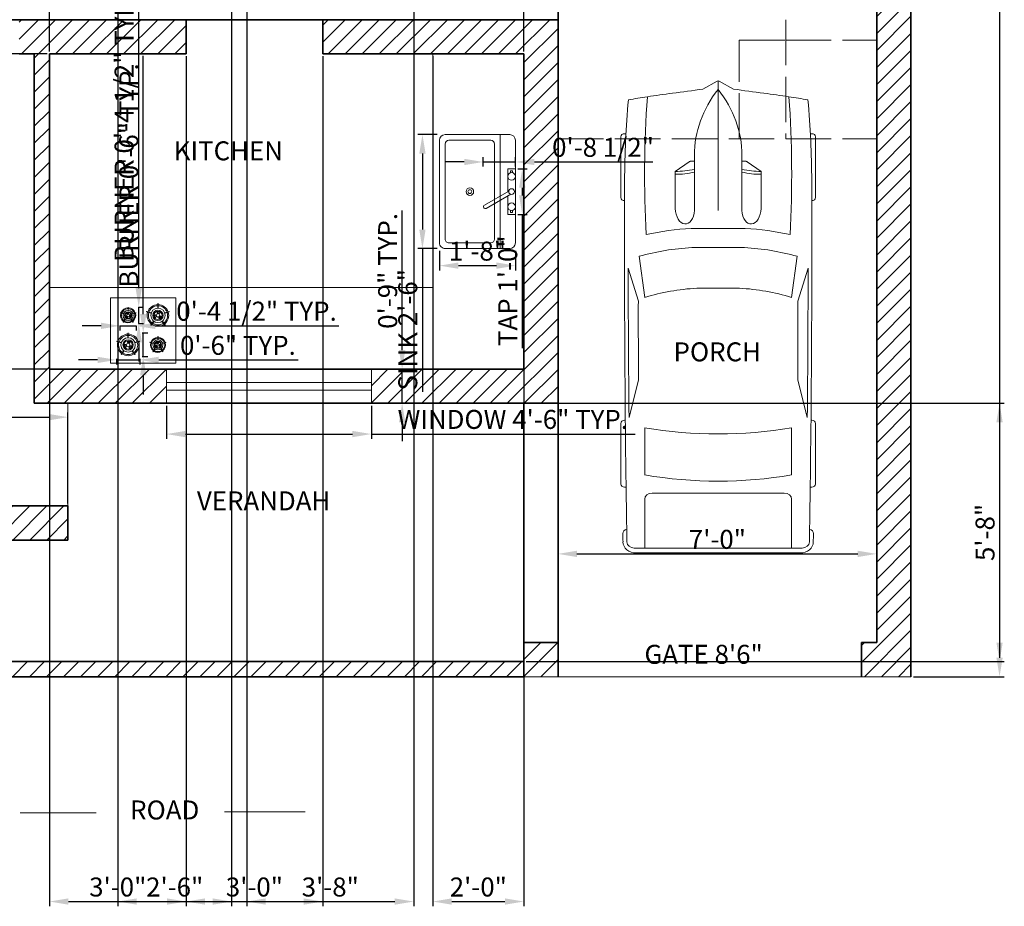
# Model space of a CAD drawing. Units: inches. Extents: x -33 to 381, y -443 to 47.
# Tile 3 of 5: x 122 to 381, y -443 to -210. Entities that reach past the tile are written whole.
import ezdxf

# ---------------------------------------------------------------- set-up
doc = ezdxf.new("R2010")
doc.units = ezdxf.units.IN
doc.linetypes.add('ACAD_ISO02W100', pattern=[15, 12, -3])
for name, color, linetype, lineweight in [('A-ANNO-DIMS', 2, 'Continuous', 18), ('A-ANNO-SYMB', 7, 'Continuous', 18), ('A-ANNO-TEXT', 7, 'Continuous', 18), ('A-AREA-IDEN', 7, 'Continuous', 18), ('A-DOOR', 4, 'Continuous', 18), ('A-EQPM', 8, 'Continuous', 15), ('A-FLOR-CASE', 9, 'Continuous', 18), ('A-FLOR-FIXT', 9, 'Continuous', 18), ('A-FLOR-STRS-OVHD', 8, 'ACAD_ISO02W100', 13), ('A-GLAZ', 4, 'Continuous', 18), ('A-SITE-VEHI', 8, 'Continuous', 13), ('A-WALL', 7, 'Continuous', 35), ('A-WALL-PATT', 251, 'Continuous', 13)]:
    doc.layers.add(name, color=color, linetype=linetype, lineweight=lineweight)
doc.styles.get("Standard").update_dxf_attribs({"font": 'arial.ttf'})
doc.dimstyles.new('ISO-25', dxfattribs={"dimtxt": 5, "dimasz": 5, "dimexe": 1.25, "dimexo": 0.625, "dimtad": 1, "dimlunit": 3, "dimtxsty": 'Standard', "dimcen": 2.5, "dimadec": 0, "dimazin": 0, "dimtfac": 1, "dimtmove": 0, "dimatfit": 3, "dimfxl": 1, "dimarcsym": 0})
pattern_1 = [(45, (-607.8963, -64.2963), (-2.245064, 2.245064), [])]

# ---------------------------------------------------------------- blocks, each defined once
blk = doc.blocks.new('Sink-single - 30 in top')
blk.add_line((-15, -3.999996), (15, -3.999996))
for points in [[(-13.5, 0), (13.5, 0)], [(-15, -18.499996), (-15, -1.5)], [(15, -1.5), (15, -18.499996)], [(-13.5, -17.499996), (-13.5, -6.499996)], [(-12.5, -5.499996), (12.5, -5.499996)], [(13.5, -6.499996), (13.5, -17.499996)], [(13.5, -19.999996), (-13.5, -19.999996)], [(12.5, -18.499996), (-12.5, -18.499996)]]:
    blk.add_lwpolyline(points)
for radius in [1, 0.5]:
    blk.add_circle((0, -11.999996), radius)
for centre, radius, start, end in [((-13.5, -1.5), 1.5, 90, 180), ((13.5, -1.5), 1.5, 0, 90), ((-12.5, -6.499996), 1, 90, 180), ((12.5, -6.499996), 1, 0, 90), ((-12.5, -17.499996), 1, 180, 270), ((12.5, -17.499996), 1, 270, 0), ((-13.5, -18.499996), 1.5, 180, 270), ((13.5, -18.499996), 1.5, 270, 0)]:
    blk.add_arc(centre, radius, start, end)
blk = doc.blocks.new('Faucet - kit sink top')
for p, q in [((-5.5, -0.75), (-5.5, -1.25)), ((-4.94278, -0.75), (-5.5, -0.75)), ((-5.5, -1.25), (-4.94278, -1.25)), ((-0.14775, -1.7441), (3.56698, -8.1782)), ((4.43301, -7.6782), (0.71828, -1.2441)), ((4.94278, -0.75), (5.5, -0.75)), ((5.5, -1.25), (4.94278, -1.25)), ((5.5, -0.75), (5.5, -1.25))]:
    blk.add_line(p, q)
blk.add_lwpolyline([(-0.00587, -2), (-6, -2), (-6, 0), (6, 0), (6, -2), (1.15195, -2)])
for centre, radius in [((-4, -1), 1), ((4, -1), 1), ((0, -1), 0.75)]:
    blk.add_circle(centre, radius)
blk.add_arc((4, -7.9282), 0.5, 210, 30)
blk = doc.blocks.new('*U10')
for p, q in [((21.1, 37.41), (21.1, 36.83)), ((46.55, 38.89), (22.35, 38.89)), ((47.8, 37.39), (47.8, 37.41)), ((87.99, 31.87), (74.76, 35.92)), ((134.31, 35.6), (119.29, 31.78)), ((135.45, 37.07), (135.45, 37.41)), ((136.7, 38.89), (160.9, 38.89)), ((162.15, 37.41), (162.15, 36.77)), ((70.03, 31.54), (86.41, 29.35)), ((186.47, -33.5), (186.47, 33.5)), ((188.4, -32.76), (188.4, 32.76)), ((138.42, 29.35), (157.25, 29.35)), ((186.47, 29.35), (167.01, 29.35)), ((164.52, 26.39), (164.52, -26.39)), ((32.27, 11.63), (36.13, 17.17)), ((36.13, 17.17), (50.94, 17.17)), ((29.77, 9.51), (51.68, 9.51)), ((32.12, 9.51), (32.12, 11.15)), ((58.92, -10.77), (58.92, 10.77)), ((66.55, -10.53), (66.55, 10.53)), ((82.74, 8.5), (82.74, -8.5)), ((186.47, -10.53), (186.47, 10.53)), ((3.27, 6.13), (0.1, 0.41)), ((0, 0), (51.68, 0)), ((0.1, -0.41), (3.27, -6.13)), ((29.77, -9.51), (51.68, -9.51)), ((32.12, -9.51), (32.12, -11.15)), ((32.27, -11.63), (36.13, -17.17)), ((36.13, -17.17), (50.94, -17.17)), ((86.41, -29.35), (70.03, -31.54)), ((157.25, -29.35), (138.42, -29.35)), ((167.01, -29.35), (186.47, -29.35)), ((87.99, -31.87), (74.76, -35.92)), ((134.31, -35.6), (119.29, -31.78)), ((21.1, -37.41), (21.1, -36.83)), ((46.55, -38.89), (22.35, -38.89)), ((47.8, -37.39), (47.8, -37.41)), ((135.45, -37.07), (135.45, -37.41)), ((136.7, -38.89), (160.9, -38.89)), ((162.15, -37.41), (162.15, -36.77))]:
    blk.add_line(p, q)
for centre, major_axis, ratio, start_param, end_param in [((266.03, -27.52), (0, 313.31), 0.842304, 1.367076, 1.39176), ((41.19, -490.86), (0, 528.23), 0.842304, 0.00281, 0.075598), ((22.35, 37.41), (0, -1.48), 0.842304, 3.141593, 4.712389), ((64.48, -10555.62), (0, 10593.03), 0.842304, -0.013397, 0.002797), ((46.55, 37.41), (0, 1.48), 0.842304, -1.570796, 0), ((64.48, -10555.62), (0, -10591.55), 0.842304, 3.133765, 3.140441), ((136.7, 37.41), (0, -1.48), 0.842304, 3.141593, 4.712389), ((160.9, 37.41), (0, 1.48), 0.842304, -1.570796, 0), ((180.63, 35.84), (0, 2.22), 0.842304, -0.013017, 1.249894), ((64.48, -10556.36), (0, 10595.31), 0.842304, -0.013397, -0.013017), ((183.98, 33.5), (0, -2.96), 0.842304, 1.570796, 3.128196), ((183.98, 32.76), (0, -5.25), 0.842304, 1.570796, 3.128196), ((135.29, 5.39), (0, 81.77), 0.842304, 1.245306, 1.50788), ((95.79, -3666.35), (0, -3698.24), 0.842304, 3.134049, 3.144098), ((259.18, -27.52), (0, -305.3), 0.842304, 4.528606, 4.561838), ((37.47, -593.96), (0, -623.33), 0.842304, 3.096046, 3.200911), ((134.4, 5.39), (0, -89.78), 0.842304, 4.449482, 4.652344), ((149.6, 2.8), (0, -79.58), 0.842304, 4.372215, 4.640744), ((17.08, 0), (0, 147.02), 0.842304, 4.511394, 4.913384), ((35.91, 0), (0, 147.02), 0.842304, 4.511394, 4.913384), ((167.01, 26.39), (0, 2.96), 0.842304, 0, 1.570796), ((-204.49, 52.4), (0, -250.96), 0.842304, 1.385369, 1.434372), ((13.04, 17.01), (0, 27.42), 0.842304, 4.435146, 4.718221), ((14.2, 17.01), (0, 27.42), 0.842304, 4.435146, 4.718221), ((50.79, 13.34), (6.34, -0.36), 0.603834, -1.395552, 1.581315), ((29.77, -46.66), (0, 56.17), 0.842304, 0, 0.590319), ((32.75, 11.15), (0, 0.74), 0.842304, 0.879714, 1.570796), ((0.62, 0), (0, -0.74), 0.842304, 4.131459, 5.293319), ((29.77, 46.66), (0, 56.17), 0.842304, 2.551274, 3.141593), ((-204.49, -52.4), (0, 250.96), 0.842304, -1.434372, -1.385369), ((32.75, -11.15), (0, -0.74), 0.842304, 4.712389, 5.403472), ((13.04, -17.01), (0, -27.42), 0.842304, 1.564964, 1.848039), ((14.2, -17.01), (0, -27.42), 0.842304, 1.564964, 1.848039), ((134.4, -5.39), (0, -89.78), 0.842304, -1.510751, -1.307889), ((135.29, -5.39), (0, -81.77), 0.842304, -1.50788, -1.245306), ((149.6, -2.8), (0, -79.58), 0.842304, -1.499151, -1.230623), ((259.18, 27.52), (0, 305.3), 0.842304, 1.721348, 1.754579), ((167.01, -26.39), (0, -2.96), 0.842304, 4.712389, 6.283185), ((266.03, 27.52), (0, 313.31), 0.842304, 1.749832, 1.774517), ((37.47, 593.96), (0, -623.33), 0.842304, -0.059319, 0.045547), ((95.79, 3666.35), (0, -3698.24), 0.842304, -0.002505, 0.007544), ((183.98, -33.5), (0, 2.96), 0.842304, 3.15499, 4.712389), ((183.98, -32.76), (0, -5.25), 0.842304, 0.013397, 1.570796), ((41.19, 490.86), (0, -528.23), 0.842304, -0.075598, -0.00281), ((22.35, -37.41), (0, 1.48), 0.842304, 1.570796, 3.141593), ((64.48, 10555.62), (0, 10593.03), 0.842304, 3.138796, 3.15499), ((46.55, -37.41), (0, -1.48), 0.842304, 0, 1.570796), ((64.48, 10555.62), (0, -10591.55), 0.842304, 0.001152, 0.007828), ((136.7, -37.41), (0, -1.48), 0.842304, -1.570796, 0), ((160.9, -37.41), (0, 1.48), 0.842304, 3.141593, 4.712389), ((180.63, -35.84), (0, -2.22), 0.842304, -1.249894, 0.013017), ((64.48, 10556.36), (0, 10595.31), 0.842304, 3.15461, 3.15499)]:
    blk.add_ellipse(centre, major_axis=major_axis, ratio=ratio, start_param=start_param, end_param=end_param)
at = {"extrusion": (0, 0, -1)}
blk.add_ellipse((50.79, -13.34), major_axis=(6.34, 0.36), ratio=0.603834, start_param=-1.395552, end_param=1.581315, dxfattribs=at)
blk = doc.blocks.new('COOKTOP-BURNER-LARGE')
for p, q in [((2.95, 4.78), (2.95, 5.94)), ((3.05, 4.78), (3.05, 5.94)), ((1.14, 3.39), (0.03, 3.75)), ((1.17, 3.48), (0.06, 3.84)), ((4.83, 3.48), (5.94, 3.84)), ((4.86, 3.39), (5.97, 3.75)), ((1.82, 1.3), (1.14, 0.35)), ((1.9, 1.24), (1.21, 0.3)), ((4.1, 1.24), (4.78, 0.3)), ((4.18, 1.3), (4.86, 0.35))]:
    blk.add_line(p, q)
for radius in [1.89, 1.36, 1.1, 0.473]:
    blk.add_circle((3, 2.84), radius)
for centre, radius, start, end in [((3, 2.84), 2.84, 90.9557, 161.0457), ((3, 2.84), 2.52, 91.075, 160.9263), ((3, 5.94), 0.0473, 0.0007, 180.0007), ((3, 2.84), 2.84, 18.9557, 89.0457), ((3, 2.84), 2.52, 19.075, 88.9263), ((0.05, 3.8), 0.0473, 72.0007, 252.0007), ((3, 2.84), 2.84, 162.9557, 233.0457), ((3, 2.84), 2.52, 163.075, 232.9263), ((1.15, 3.44), 0.0473, 252.0007, 72.0007), ((2.21, 2.84), 0.158, 0.0007, 180.0007), ((3, 2.84), 0.946, 180.0007, 213.5265), ((3, 2.84), 0.631, 180.0007, 213.5265), ((2.95, 3.62), 0.158, 93.5265, 273.5265), ((3, 2.84), 0.946, 60.0007, 93.5265), ((3, 4.78), 0.0473, 180.0007, 0.0007), ((3, 2.84), 0.631, 60.0007, 93.5265), ((3.39, 3.52), 0.158, 240.0007, 60.0007), ((3.7, 2.49), 0.158, 333.5265, 153.5265), ((3, 2.84), 2.52, 307.075, 16.9263), ((3, 2.84), 2.84, 306.9557, 17.0457), ((4.84, 3.44), 0.0473, 108.0007, 288.0007), ((5.95, 3.8), 0.0473, 288.0007, 108.0007), ((1.17, 0.33), 0.0473, 144.0007, 324.0007), ((3, 2.84), 2.84, 234.9557, 305.0457), ((3, 2.84), 2.52, 235.075, 304.9263), ((1.86, 1.27), 0.0473, 324.0007, 144.0007), ((2.34, 2.4), 0.158, 213.5265, 33.5265), ((3.39, 2.16), 0.158, 120.0007, 300.0007), ((3, 2.84), 0.631, 300.0007, 333.5265), ((3, 2.84), 0.946, 300.0007, 333.5265), ((4.14, 1.27), 0.0473, 36.0007, 216.0007), ((4.82, 0.33), 0.0473, 216.0007, 36.0007)]:
    blk.add_arc(centre, radius, start, end)
blk = doc.blocks.new('COOKTOP-BURNER-SMALL')
for p, q in [((0.8, 2.37), (0.02, 2.63)), ((0.82, 2.44), (0.04, 2.69)), ((2.07, 3.34), (2.07, 4.16)), ((2.13, 3.34), (2.13, 4.16)), ((3.38, 2.44), (4.15, 2.69)), ((3.4, 2.37), (4.18, 2.63)), ((1.27, 0.91), (0.8, 0.25)), ((1.33, 0.87), (0.85, 0.21)), ((2.87, 0.87), (3.35, 0.21)), ((2.92, 0.91), (3.4, 0.25))]:
    blk.add_line(p, q)
for radius in [1.32, 0.949, 0.772, 0.331]:
    blk.add_circle((2.1, 1.99), radius)
for centre, radius, start, end in [((0.03, 2.66), 0.0331, 72.0007, 252.0007), ((2.1, 1.99), 1.99, 90.9557, 161.0457), ((2.1, 1.99), 1.77, 91.075, 160.9263), ((2.1, 1.99), 0.662, 86.4748, 120.0007), ((2.1, 4.16), 0.0331, 0.0007, 180.0007), ((2.1, 3.34), 0.0331, 180.0007, 0.0007), ((2.1, 1.99), 1.99, 18.9557, 89.0457), ((2.1, 1.99), 1.77, 19.075, 88.9263), ((2.13, 2.54), 0.11, 266.4748, 86.4748), ((4.17, 2.66), 0.0331, 288.0007, 108.0007), ((2.1, 1.99), 1.99, 162.9557, 233.0457), ((2.1, 1.99), 1.77, 163.075, 232.9263), ((0.82, 0.23), 0.0331, 144.0007, 324.0007), ((0.81, 2.41), 0.0331, 252.0007, 72.0007), ((2.02, 1.99), 1.99, 234.9557, 305.0457), ((2.1, 1.99), 1.77, 235.075, 304.9263), ((1.3, 0.89), 0.0331, 324.0007, 144.0007), ((1.61, 1.74), 0.11, 26.4748, 206.4748), ((2.1, 1.99), 0.662, 206.4748, 240.0007), ((2.1, 1.99), 0.441, 206.4748, 240.0007), ((1.82, 2.46), 0.11, 120.0007, 300.0007), ((1.82, 1.51), 0.11, 240.0007, 60.0007), ((2.1, 1.99), 0.441, 86.4748, 120.0007), ((2.56, 1.68), 0.11, 146.4748, 326.4748), ((2.1, 1.99), 0.441, 326.4748, 0.0007), ((2.65, 1.99), 0.11, 0.0007, 180.0007), ((2.1, 1.99), 0.662, 326.4748, 0.0007), ((2.9, 0.89), 0.0331, 36.0007, 216.0007), ((2.1, 1.99), 1.77, 307.075, 16.9263), ((2.1, 1.99), 1.99, 306.9557, 17.0457), ((3.38, 0.23), 0.0331, 216.0007, 36.0007), ((3.39, 2.41), 0.0331, 108.0007, 288.0007)]:
    blk.add_arc(centre, radius, start, end)
blk = doc.blocks.new('WINDOW-54IN')
for p, q in [((0, 5.5), (54, 5.5)), ((0, 3.5), (54, 3.5))]:
    blk.add_line(p, q)
blk.add_lwpolyline([(0, 9), (54, 9), (54, 0), (0, 0)], close=True)
blk = doc.blocks.new('*D27')
at = {"layer": 'A-ANNO-DIMS', "color": 0, "lineweight": -2, "transparency": 16777216}
for p, q in [((160.37, -311.45), (160.37, -320.17)), ((214.37, -311.45), (214.37, -320.17)), ((165.37, -318.92), (209.37, -318.92)), ((214.37, -318.92), (283.9, -318.92))]:
    blk.add_line(p, q, dxfattribs=at)
at = {"layer": 'A-ANNO-DIMS', "color": 0, "transparency": 16777216}
for points in [[(165.37, -318.09), (165.37, -319.75), (160.37, -318.92)], [(209.37, -318.09), (209.37, -319.75), (214.37, -318.92)]]:
    blk.add_solid(points, dxfattribs=at)
at = {"layer": 'Defpoints', "color": 0, "transparency": 16777216}
for p in [(160.37, -310.82), (214.37, -310.82), (214.37, -318.92)]:
    blk.add_point(p, dxfattribs=at)
at = {"layer": 'A-ANNO-DIMS', "color": 0, "transparency": 16777216, "insert": (251.63, -315.71), "char_height": 5, "attachment_point": 5}
blk.add_mtext('WINDOW 4\'-6" TYP.', dxfattribs=at)
blk = doc.blocks.new('*D28')
at = {"layer": 'A-ANNO-DIMS', "color": 0, "lineweight": -2, "transparency": 16777216}
for p, q in [((222.47, -296.82), (222.47, -260.09)), ((215, -301.82), (223.72, -301.82)), ((222.47, -310.82), (222.47, -301.82)), ((215, -310.82), (223.72, -310.82)), ((222.47, -315.82), (222.47, -320.82))]:
    blk.add_line(p, q, dxfattribs=at)
at = {"layer": 'A-ANNO-DIMS', "color": 0, "transparency": 16777216}
for points in [[(221.64, -296.82), (223.31, -296.82), (222.47, -301.82)], [(221.64, -315.82), (223.31, -315.82), (222.47, -310.82)]]:
    blk.add_solid(points, dxfattribs=at)
at = {"layer": 'Defpoints', "color": 0, "transparency": 16777216}
for p in [(214.37, -301.82), (222.47, -301.82), (214.37, -310.82)]:
    blk.add_point(p, dxfattribs=at)
at = {"layer": 'A-ANNO-DIMS', "color": 0, "transparency": 16777216, "insert": (219.3, -275.96), "char_height": 5, "attachment_point": 5, "rotation": 90}
blk.add_mtext('0\'-9" TYP.', dxfattribs=at)
blk = doc.blocks.new('*D31')
at = {"layer": 'A-ANNO-DIMS', "color": 0, "lineweight": -2, "transparency": 16777216}
for p, q in [((231.69, -240.08), (226.57, -240.08)), ((227.82, -245.08), (227.82, -265.08)), ((231.69, -270.08), (226.57, -270.08)), ((227.82, -270.08), (227.82, -307.84))]:
    blk.add_line(p, q, dxfattribs=at)
at = {"layer": 'A-ANNO-DIMS', "color": 0, "transparency": 16777216}
for points in [[(226.98, -245.08), (228.65, -245.08), (227.82, -240.08)], [(226.98, -265.08), (228.65, -265.08), (227.82, -270.08)]]:
    blk.add_solid(points, dxfattribs=at)
at = {"layer": 'Defpoints', "color": 0, "transparency": 16777216}
for p in [(232.32, -240.08), (227.82, -270.08), (232.32, -270.08)]:
    blk.add_point(p, dxfattribs=at)
at = {"layer": 'A-ANNO-DIMS', "color": 0, "transparency": 16777216, "insert": (224.6, -291.46), "char_height": 5, "attachment_point": 5, "rotation": 90}
blk.add_mtext('SINK 2\'-6"', dxfattribs=at)
blk = doc.blocks.new('*D32')
at = {"layer": 'A-ANNO-DIMS', "color": 0, "lineweight": -2, "transparency": 16777216}
for p, q in [((232.32, -270.7), (232.32, -275.83)), ((252.32, -270.7), (252.32, -275.83)), ((237.32, -274.58), (247.32, -274.58))]:
    blk.add_line(p, q, dxfattribs=at)
at = {"layer": 'A-ANNO-DIMS', "color": 0, "transparency": 16777216}
for points in [[(237.32, -273.74), (237.32, -275.41), (232.32, -274.58)], [(247.32, -273.74), (247.32, -275.41), (252.32, -274.58)]]:
    blk.add_solid(points, dxfattribs=at)
at = {"layer": 'Defpoints', "color": 0, "transparency": 16777216}
for p in [(232.32, -270.08), (252.32, -270.08), (252.32, -274.58)]:
    blk.add_point(p, dxfattribs=at)
at = {"layer": 'A-ANNO-DIMS', "color": 0, "transparency": 16777216, "insert": (242.32, -271.4), "char_height": 5, "attachment_point": 5}
blk.add_mtext('1\'-8"', dxfattribs=at)
blk = doc.blocks.new('*D33')
at = {"layer": 'A-ANNO-DIMS', "color": 0, "lineweight": -2, "transparency": 16777216}
for p, q in [((252.94, -249.08), (255.37, -249.08)), ((254.12, -254.08), (254.12, -256.08)), ((252.94, -261.08), (255.37, -261.08)), ((254.12, -261.08), (254.12, -296.27))]:
    blk.add_line(p, q, dxfattribs=at)
at = {"layer": 'A-ANNO-DIMS', "color": 0, "transparency": 16777216}
for points in [[(253.28, -254.08), (254.95, -254.08), (254.12, -249.08)], [(253.28, -256.08), (254.95, -256.08), (254.12, -261.08)]]:
    blk.add_solid(points, dxfattribs=at)
at = {"layer": 'Defpoints', "color": 0, "transparency": 16777216}
for p in [(252.32, -249.08), (252.32, -261.08), (254.12, -261.08)]:
    blk.add_point(p, dxfattribs=at)
at = {"layer": 'A-ANNO-DIMS', "color": 0, "transparency": 16777216, "insert": (250.94, -281.17), "char_height": 5, "attachment_point": 5, "rotation": 90}
blk.add_mtext('TAP 1\'-0"', dxfattribs=at)
blk = doc.blocks.new('*D34')
at = {"layer": 'A-ANNO-DIMS', "color": 0, "lineweight": -2, "transparency": 16777216}
for p, q in [((243.82, -248.45), (243.82, -246.03)), ((252.32, -248.45), (252.32, -246.03)), ((238.82, -247.28), (233.82, -247.28)), ((243.82, -247.28), (252.32, -247.28)), ((257.32, -247.28), (288.51, -247.28))]:
    blk.add_line(p, q, dxfattribs=at)
at = {"layer": 'A-ANNO-DIMS', "color": 0, "transparency": 16777216}
for points in [[(238.82, -246.44), (238.82, -248.11), (243.82, -247.28)], [(257.32, -246.44), (257.32, -248.11), (252.32, -247.28)]]:
    blk.add_solid(points, dxfattribs=at)
at = {"layer": 'Defpoints', "color": 0, "transparency": 16777216}
for p in [(252.32, -247.28), (243.82, -249.08), (252.32, -249.08)]:
    blk.add_point(p, dxfattribs=at)
at = {"layer": 'A-ANNO-DIMS', "color": 0, "transparency": 16777216, "insert": (275.41, -244.07), "char_height": 5, "attachment_point": 5}
blk.add_mtext('0\'-8 1/2"', dxfattribs=at)
blk = doc.blocks.new('*D35')
at = {"layer": 'A-ANNO-DIMS', "color": 0, "lineweight": -2, "transparency": 16777216}
for p, q in [((153.06, -280.47), (153.06, -200.88)), ((153.04, -285.47), (154.31, -285.47)), ((153.06, -289.78), (153.06, -285.47)), ((153.04, -289.78), (154.31, -289.78)), ((153.06, -294.78), (153.06, -299.78))]:
    blk.add_line(p, q, dxfattribs=at)
at = {"layer": 'A-ANNO-DIMS', "color": 0, "transparency": 16777216}
for points in [[(152.22, -280.47), (153.89, -280.47), (153.06, -285.47)], [(152.22, -294.78), (153.89, -294.78), (153.06, -289.78)]]:
    blk.add_solid(points, dxfattribs=at)
at = {"layer": 'Defpoints', "color": 0, "transparency": 16777216}
for p in [(152.41, -285.47), (153.06, -285.47), (152.41, -289.78)]:
    blk.add_point(p, dxfattribs=at)
at = {"layer": 'A-ANNO-DIMS', "color": 0, "transparency": 16777216, "insert": (149.85, -238.18), "char_height": 5, "attachment_point": 5, "rotation": 90}
blk.add_mtext('BURNER 0\'-4 1/2" TYP.', dxfattribs=at)
blk = doc.blocks.new('*D36')
at = {"layer": 'A-ANNO-DIMS', "color": 0, "lineweight": -2, "transparency": 16777216}
for p, q in [((143.12, -290.43), (138.12, -290.43)), ((148.12, -290.41), (148.12, -291.68)), ((148.12, -290.43), (152.41, -290.43)), ((152.41, -290.41), (152.41, -291.68)), ((157.41, -290.43), (205.79, -290.43))]:
    blk.add_line(p, q, dxfattribs=at)
at = {"layer": 'A-ANNO-DIMS', "color": 0, "transparency": 16777216}
for points in [[(143.12, -289.6), (143.12, -291.26), (148.12, -290.43)], [(157.41, -289.6), (157.41, -291.26), (152.41, -290.43)]]:
    blk.add_solid(points, dxfattribs=at)
at = {"layer": 'Defpoints', "color": 0, "transparency": 16777216}
for p in [(148.12, -289.78), (152.41, -289.78), (152.41, -290.43)]:
    blk.add_point(p, dxfattribs=at)
at = {"layer": 'A-ANNO-DIMS', "color": 0, "transparency": 16777216, "insert": (184.1, -287.22), "char_height": 5, "attachment_point": 5}
blk.add_mtext('0\'-4 1/2" TYP.', dxfattribs=at)
blk = doc.blocks.new('*D37')
at = {"layer": 'A-ANNO-DIMS', "color": 0, "lineweight": -2, "transparency": 16777216}
for p, q in [((154.25, -287.31), (154.25, -219.36)), ((153.96, -292.31), (155.5, -292.31)), ((154.25, -298.47), (154.25, -292.31)), ((153.96, -298.47), (155.5, -298.47)), ((154.25, -303.47), (154.25, -308.47))]:
    blk.add_line(p, q, dxfattribs=at)
at = {"layer": 'A-ANNO-DIMS', "color": 0, "transparency": 16777216}
for points in [[(153.42, -287.31), (155.09, -287.31), (154.25, -292.31)], [(153.42, -303.47), (155.09, -303.47), (154.25, -298.47)]]:
    blk.add_solid(points, dxfattribs=at)
at = {"layer": 'Defpoints', "color": 0, "transparency": 16777216}
for p in [(153.33, -292.31), (154.25, -292.31), (153.33, -298.47)]:
    blk.add_point(p, dxfattribs=at)
at = {"layer": 'A-ANNO-DIMS', "color": 0, "transparency": 16777216, "insert": (151.08, -250.83), "char_height": 5, "attachment_point": 5, "rotation": 90}
blk.add_mtext('BURNER 0\'-6" TYP.', dxfattribs=at)
blk = doc.blocks.new('*D38')
at = {"layer": 'A-ANNO-DIMS', "color": 0, "lineweight": -2, "transparency": 16777216}
for p, q in [((142.2, -299.39), (137.2, -299.39)), ((147.2, -299.09), (147.2, -300.64)), ((147.2, -299.39), (153.33, -299.39)), ((153.33, -299.09), (153.33, -300.64)), ((158.33, -299.39), (195.06, -299.39))]:
    blk.add_line(p, q, dxfattribs=at)
at = {"layer": 'A-ANNO-DIMS', "color": 0, "transparency": 16777216}
for points in [[(142.2, -298.56), (142.2, -300.22), (147.2, -299.39)], [(158.33, -298.56), (158.33, -300.22), (153.33, -299.39)]]:
    blk.add_solid(points, dxfattribs=at)
at = {"layer": 'Defpoints', "color": 0, "transparency": 16777216}
for p in [(147.2, -298.47), (153.33, -298.47), (153.33, -299.39)]:
    blk.add_point(p, dxfattribs=at)
at = {"layer": 'A-ANNO-DIMS', "color": 0, "transparency": 16777216, "insert": (179.19, -296.21), "char_height": 5, "attachment_point": 5}
blk.add_mtext('0\'-6" TYP.', dxfattribs=at)
blk = doc.blocks.new('*D39')
at = {"layer": 'A-ANNO-DIMS', "color": 0, "lineweight": -2, "transparency": 16777216}
for p, q in [((357.17, 13.18), (381.14, 13.18)), ((379.89, 8.18), (379.89, -377.82)), ((357.17, -382.82), (381.14, -382.82))]:
    blk.add_line(p, q, dxfattribs=at)
at = {"layer": 'A-ANNO-DIMS', "color": 0, "transparency": 16777216}
for points in [[(379.06, 8.18), (380.72, 8.18), (379.89, 13.18)], [(379.06, -377.82), (380.72, -377.82), (379.89, -382.82)]]:
    blk.add_solid(points, dxfattribs=at)
at = {"layer": 'Defpoints', "color": 0, "transparency": 16777216}
for p in [(356.54, 13.18), (356.54, -382.82), (379.89, -382.82)]:
    blk.add_point(p, dxfattribs=at)
at = {"layer": 'A-ANNO-DIMS', "color": 0, "transparency": 16777216, "insert": (376.71, -184.82), "char_height": 5, "attachment_point": 5, "rotation": 90}
blk.add_mtext('33\'-0"', dxfattribs=at)
blk = doc.blocks.new('*D47')
at = {"layer": 'A-ANNO-DIMS', "color": 0, "lineweight": -2, "transparency": 16777216}
for p, q in [((129.54, -218.2), (129.54, 37.78)), ((134.54, 36.53), (249.54, 36.53)), ((254.54, -218.2), (254.54, 37.78))]:
    blk.add_line(p, q, dxfattribs=at)
at = {"layer": 'A-ANNO-DIMS', "color": 0, "transparency": 16777216}
for points in [[(134.54, 37.36), (134.54, 35.7), (129.54, 36.53)], [(249.54, 37.36), (249.54, 35.7), (254.54, 36.53)]]:
    blk.add_solid(points, dxfattribs=at)
at = {"layer": 'Defpoints', "color": 0, "transparency": 16777216}
for p in [(254.54, 36.53), (129.54, -218.82), (254.54, -218.82)]:
    blk.add_point(p, dxfattribs=at)
at = {"layer": 'A-ANNO-DIMS', "color": 0, "transparency": 16777216, "insert": (192.04, 39.71), "char_height": 5, "attachment_point": 5}
blk.add_mtext('10\'-5"', dxfattribs=at)
blk = doc.blocks.new('*D48')
at = {"layer": 'A-ANNO-DIMS', "color": 0, "lineweight": -2, "transparency": 16777216}
for p, q in [((128.92, -218.82), (-28.06, -218.82)), ((-26.81, -223.82), (-26.81, -296.82)), ((128.92, -301.82), (-28.06, -301.82))]:
    blk.add_line(p, q, dxfattribs=at)
at = {"layer": 'A-ANNO-DIMS', "color": 0, "transparency": 16777216}
for points in [[(-27.64, -223.82), (-25.98, -223.82), (-26.81, -218.82)], [(-27.64, -296.82), (-25.98, -296.82), (-26.81, -301.82)]]:
    blk.add_solid(points, dxfattribs=at)
at = {"layer": 'Defpoints', "color": 0, "transparency": 16777216}
for p in [(129.54, -218.82), (-26.81, -301.82), (129.54, -301.82)]:
    blk.add_point(p, dxfattribs=at)
at = {"layer": 'A-ANNO-DIMS', "color": 0, "transparency": 16777216, "insert": (-29.99, -260.32), "char_height": 5, "attachment_point": 5, "rotation": 90}
blk.add_mtext('6\'-11"', dxfattribs=at)
blk = doc.blocks.new('*D52')
at = {"layer": 'A-ANNO-DIMS', "color": 0, "lineweight": -2, "transparency": 16777216}
for p, q in [((181.54, -125.45), (181.54, -443.26)), ((225.54, -125.45), (225.54, -443.26)), ((186.54, -442.01), (220.54, -442.01))]:
    blk.add_line(p, q, dxfattribs=at)
at = {"layer": 'A-ANNO-DIMS', "color": 0, "transparency": 16777216}
for points in [[(186.54, -441.18), (186.54, -442.84), (181.54, -442.01)], [(220.54, -441.18), (220.54, -442.84), (225.54, -442.01)]]:
    blk.add_solid(points, dxfattribs=at)
at = {"layer": 'Defpoints', "color": 0, "transparency": 16777216}
for p in [(181.54, -124.82), (225.54, -124.82), (225.54, -442.01)]:
    blk.add_point(p, dxfattribs=at)
at = {"layer": 'A-ANNO-DIMS', "color": 0, "transparency": 16777216, "insert": (203.54, -438.83), "char_height": 5, "attachment_point": 5}
blk.add_mtext('3\'-8"', dxfattribs=at)
blk = doc.blocks.new('*D55')
at = {"layer": 'A-ANNO-DIMS', "color": 0, "lineweight": -2, "transparency": 16777216}
for p, q in [((263.54, -373.2), (263.54, -349.22)), ((347.54, -373.2), (347.54, -349.22)), ((268.54, -350.47), (342.54, -350.47))]:
    blk.add_line(p, q, dxfattribs=at)
at = {"layer": 'A-ANNO-DIMS', "color": 0, "transparency": 16777216}
for points in [[(268.54, -349.64), (268.54, -351.3), (263.54, -350.47)], [(342.54, -349.64), (342.54, -351.3), (347.54, -350.47)]]:
    blk.add_solid(points, dxfattribs=at)
at = {"layer": 'Defpoints', "color": 0, "transparency": 16777216}
for p in [(347.54, -350.47), (263.54, -373.82), (347.54, -373.82)]:
    blk.add_point(p, dxfattribs=at)
at = {"layer": 'A-ANNO-DIMS', "color": 0, "transparency": 16777216, "insert": (305.54, -347.29), "char_height": 5, "attachment_point": 5}
blk.add_mtext('7\'-0"', dxfattribs=at)
blk = doc.blocks.new('*D56')
at = {"layer": 'A-ANNO-DIMS', "color": 0, "lineweight": -2, "transparency": 16777216}
for p, q in [((255.17, -310.82), (381.14, -310.82)), ((379.89, -315.82), (379.89, -373.82)), ((255.17, -378.82), (381.14, -378.82))]:
    blk.add_line(p, q, dxfattribs=at)
at = {"layer": 'A-ANNO-DIMS', "color": 0, "transparency": 16777216}
for points in [[(379.06, -315.82), (380.72, -315.82), (379.89, -310.82)], [(379.06, -373.82), (380.72, -373.82), (379.89, -378.82)]]:
    blk.add_solid(points, dxfattribs=at)
at = {"layer": 'Defpoints', "color": 0, "transparency": 16777216}
for p in [(254.54, -310.82), (254.54, -378.82), (379.89, -378.82)]:
    blk.add_point(p, dxfattribs=at)
at = {"layer": 'A-ANNO-DIMS', "color": 0, "transparency": 16777216, "insert": (376.71, -344.82), "char_height": 5, "attachment_point": 5, "rotation": 90}
blk.add_mtext('5\'-8"', dxfattribs=at)
blk = doc.blocks.new('*D58')
at = {"layer": 'A-ANNO-DIMS', "color": 0, "lineweight": -2, "transparency": 16777216}
for p, q in [((230.54, -219.45), (230.54, -443.26)), ((254.54, -219.45), (254.54, -443.26)), ((235.54, -442.01), (249.54, -442.01))]:
    blk.add_line(p, q, dxfattribs=at)
at = {"layer": 'A-ANNO-DIMS', "color": 0, "transparency": 16777216}
for points in [[(235.54, -441.18), (235.54, -442.84), (230.54, -442.01)], [(249.54, -441.18), (249.54, -442.84), (254.54, -442.01)]]:
    blk.add_solid(points, dxfattribs=at)
at = {"layer": 'Defpoints', "color": 0, "transparency": 16777216}
for p in [(230.54, -218.82), (254.54, -218.82), (254.54, -442.01)]:
    blk.add_point(p, dxfattribs=at)
at = {"layer": 'A-ANNO-DIMS', "color": 0, "transparency": 16777216, "insert": (242.54, -438.83), "char_height": 5, "attachment_point": 5}
blk.add_mtext('2\'-0"', dxfattribs=at)
blk = doc.blocks.new('*D59')
at = {"layer": 'A-ANNO-DIMS', "color": 0, "lineweight": -2, "transparency": 16777216}
for p, q in [((165.54, -219.45), (165.54, -443.26)), ((201.54, -219.45), (201.54, -443.26)), ((170.54, -442.01), (196.54, -442.01))]:
    blk.add_line(p, q, dxfattribs=at)
at = {"layer": 'A-ANNO-DIMS', "color": 0, "transparency": 16777216}
for points in [[(170.54, -441.18), (170.54, -442.84), (165.54, -442.01)], [(196.54, -441.18), (196.54, -442.84), (201.54, -442.01)]]:
    blk.add_solid(points, dxfattribs=at)
at = {"layer": 'Defpoints', "color": 0, "transparency": 16777216}
for p in [(165.54, -218.82), (201.54, -218.82), (201.54, -442.01)]:
    blk.add_point(p, dxfattribs=at)
at = {"layer": 'A-ANNO-DIMS', "color": 0, "transparency": 16777216, "insert": (183.54, -438.83), "char_height": 5, "attachment_point": 5}
blk.add_mtext('3\'-0"', dxfattribs=at)
blk = doc.blocks.new('*D60')
at = {"layer": 'A-ANNO-DIMS', "color": 0, "lineweight": -2, "transparency": 16777216}
for p, q in [((129.54, -219.45), (129.54, -443.26)), ((165.54, -219.45), (165.54, -443.26)), ((134.54, -442.01), (160.54, -442.01))]:
    blk.add_line(p, q, dxfattribs=at)
at = {"layer": 'A-ANNO-DIMS', "color": 0, "transparency": 16777216}
for points in [[(134.54, -441.18), (134.54, -442.84), (129.54, -442.01)], [(160.54, -441.18), (160.54, -442.84), (165.54, -442.01)]]:
    blk.add_solid(points, dxfattribs=at)
at = {"layer": 'Defpoints', "color": 0, "transparency": 16777216}
for p in [(129.54, -218.82), (165.54, -218.82), (165.54, -442.01)]:
    blk.add_point(p, dxfattribs=at)
at = {"layer": 'A-ANNO-DIMS', "color": 0, "transparency": 16777216, "insert": (147.54, -438.83), "char_height": 5, "attachment_point": 5}
blk.add_mtext('3\'-0"', dxfattribs=at)
blk = doc.blocks.new('*D61')
at = {"layer": 'A-ANNO-DIMS', "color": 0, "lineweight": -2, "transparency": 16777216}
for p, q in [((147.54, -77.49), (147.54, -443.26)), ((177.54, -77.49), (177.54, -443.26)), ((152.54, -442.01), (172.54, -442.01))]:
    blk.add_line(p, q, dxfattribs=at)
at = {"layer": 'A-ANNO-DIMS', "color": 0, "transparency": 16777216}
for points in [[(152.54, -441.18), (152.54, -442.84), (147.54, -442.01)], [(172.54, -441.18), (172.54, -442.84), (177.54, -442.01)]]:
    blk.add_solid(points, dxfattribs=at)
at = {"layer": 'Defpoints', "color": 0, "transparency": 16777216}
for p in [(147.54, -76.86), (177.54, -76.86), (177.54, -442.01)]:
    blk.add_point(p, dxfattribs=at)
at = {"layer": 'A-ANNO-DIMS', "color": 0, "transparency": 16777216, "insert": (162.54, -438.83), "char_height": 5, "attachment_point": 5}
blk.add_mtext('2\'-6"', dxfattribs=at)
blk = doc.blocks.new('*D63')
at = {"layer": 'A-ANNO-DIMS', "color": 0, "lineweight": -2, "transparency": 16777216}
for p, q in [((5.54, -337.2), (5.54, -313.22)), ((134.42, -337.2), (134.42, -313.22)), ((10.54, -314.47), (129.42, -314.47))]:
    blk.add_line(p, q, dxfattribs=at)
at = {"layer": 'A-ANNO-DIMS', "color": 0, "transparency": 16777216}
for points in [[(10.54, -313.64), (10.54, -315.3), (5.54, -314.47)], [(129.42, -313.64), (129.42, -315.3), (134.42, -314.47)]]:
    blk.add_solid(points, dxfattribs=at)
at = {"layer": 'Defpoints', "color": 0, "transparency": 16777216}
for p in [(134.42, -314.47), (5.54, -337.82), (134.42, -337.82)]:
    blk.add_point(p, dxfattribs=at)
at = {"layer": 'A-ANNO-DIMS', "color": 0, "transparency": 16777216, "insert": (69.98, -311.29), "char_height": 5, "attachment_point": 5}
blk.add_mtext('10\'-9"', dxfattribs=at)

msp = doc.modelspace()

# ---------------------------------------------------------------- hatches: boundary and pattern name
at = {"layer": 'A-WALL-PATT'}
h = msp.add_hatch(dxfattribs=at)
h.set_pattern_fill('ANSI31', color=256)
h.set_pattern_definition(pattern_1)
h.paths.add_polyline_path([(356.541, 13.18), (-3.459, 13.18), (-3.459, -346.82), (-3.459, -382.82), (254.541, -382.82), (254.541, -378.82), (5.541, -378.82), (5.541, -346.82), (36.25, -346.82), (36.25, -337.82), (5.541, -337.82), (5.541, 4.18), (125.541, 4.18), (125.541, -123.82), (129.541, -123.82), (129.541, -76.862), (147.541, -76.862), (147.541, -72.862), (129.541, -72.862), (129.541, 4.18), (225.541, 4.18), (225.541, -124.82), (181.541, -124.82), (181.541, -120.82), (177.541, -120.82), (177.541, -128.82), (229.541, -128.82), (229.541, 4.18), (347.541, 4.18), (347.541, -119.82), (329.098, -119.82), (329.098, -128.82), (347.541, -128.82), (347.541, -373.82), (343.541, -373.82), (343.541, -382.82), (356.541, -382.82), (356.541, -346.82)])
h.paths.add_polyline_path([(181.541, -35.82), (188.17, -35.82), (188.17, -31.82), (172.2, -31.82), (172.2, -35.82), (177.541, -35.82), (177.541, -90.82), (181.541, -90.82)], flags=17)
h.paths.add_polyline_path([(225.541, -31.82), (222.17, -31.82), (222.17, -35.82), (225.541, -35.82)], flags=17)
h.paths.add_polyline_path([(138.2, -31.82), (129.541, -31.82), (129.541, -35.82), (138.2, -35.82)], flags=17)
h.paths.add_polyline_path([(89.541, -167.82), (85.541, -167.82), (85.541, -209.82), (5.541, -209.82), (5.541, -218.82), (90.906, -218.82), (90.906, -209.82), (89.541, -209.82)], flags=17)
h.paths.add_polyline_path([(165.541, -209.82), (125.541, -209.82), (121.541, -209.82), (121.541, -218.82), (125.541, -218.82), (125.541, -310.82), (160.374, -310.82), (160.374, -301.82), (129.541, -301.82), (129.541, -218.82), (165.541, -218.82)], flags=17)
h.paths.add_polyline_path([(263.541, -209.82), (254.541, -209.82), (201.541, -209.82), (201.541, -218.82), (254.541, -218.82), (254.541, -301.82), (214.374, -301.82), (214.374, -310.82), (254.541, -310.82), (263.541, -310.82)], flags=17)
h.paths.add_polyline_path([(263.541, -128.82), (275.098, -128.82), (275.098, -119.82), (254.541, -119.82), (254.541, -128.82), (254.541, -165.974), (263.541, -165.974)], flags=17)
h.paths.add_polyline_path([(263.541, -373.82), (254.541, -373.82), (254.541, -382.82), (263.541, -382.82)], flags=17)
h = msp.add_hatch(dxfattribs=at)
h.set_pattern_fill('ANSI31', color=256)
h.set_pattern_definition(pattern_1)
h.paths.add_polyline_path([(134.422, -337.82), (90.25, -337.82), (90.25, -346.82), (134.422, -346.82)])

# ---------------------------------------------------------------- linework, layer by layer
at = {"layer": 'A-ANNO-SYMB'}
for p, q in [((141.865, -418.659), (121.847, -418.659)), ((175.618, -418.427), (196.917, -418.427))]:
    msp.add_line(p, q, dxfattribs=at)
at = {"layer": 'A-DOOR'}
for p, q in [((134.422, -337.82), (134.422, -310.82)), ((254.541, -382.82), (356.541, -382.82))]:
    msp.add_line(p, q, dxfattribs=at)
at = {"layer": 'A-EQPM'}
msp.add_lwpolyline([(145.598, -300.217), (162.796, -300.217), (162.796, -283.019), (145.598, -283.019)], close=True, dxfattribs=at)
at = {"layer": 'A-FLOR-CASE'}
for p, q in [((230.541, -218.82), (230.541, -280.289)), ((230.541, -280.289), (129.541, -280.289))]:
    msp.add_line(p, q, dxfattribs=at)
at = {"layer": 'A-FLOR-STRS-OVHD'}
for p, q in [((323.541, -164.82), (323.541, -241.188)), ((311.297, -241.188), (311.297, -215.176)), ((311.297, -215.176), (323.541, -215.176)), ((323.541, -215.176), (347.541, -215.176)), ((263.541, -241.188), (347.541, -241.188))]:
    msp.add_line(p, q, dxfattribs=at)
at = {"layer": 'A-WALL'}
for p, q in [((356.541, 13.18), (356.541, -346.82)), ((263.541, -128.82), (263.541, -310.82)), ((347.541, -128.82), (347.541, -373.82)), ((89.541, -209.82), (125.541, -209.82)), ((125.541, -209.82), (254.541, -209.82)), ((165.541, -209.82), (165.541, -218.82)), ((201.541, -209.82), (201.541, -218.82)), ((254.541, -209.82), (263.541, -209.82)), ((121.541, -218.82), (125.541, -218.82)), ((125.541, -310.82), (125.541, -218.82)), ((129.541, -301.82), (129.541, -218.82)), ((129.541, -218.82), (165.541, -218.82)), ((201.541, -218.82), (254.541, -218.82)), ((254.541, -218.82), (254.541, -301.82)), ((129.541, -301.82), (254.541, -301.82)), ((125.541, -310.82), (254.541, -310.82)), ((254.541, -310.82), (263.541, -310.82)), ((254.541, -310.82), (254.541, -382.82)), ((263.541, -310.82), (263.541, -382.82)), ((134.422, -337.82), (5.541, -337.82)), ((134.422, -337.82), (134.422, -346.82)), ((134.422, -346.82), (5.541, -346.82)), ((356.541, -382.82), (356.541, -346.82)), ((254.541, -373.82), (263.541, -373.82)), ((343.541, -373.82), (343.541, -382.82)), ((343.541, -373.82), (347.541, -373.82)), ((5.541, -378.82), (254.541, -378.82)), ((-3.459, -382.82), (254.541, -382.82))]:
    msp.add_line(p, q, dxfattribs=at)

# ---------------------------------------------------------------- block references
at = {"layer": 'A-EQPM'}
for name, p in [('COOKTOP-BURNER-LARGE', (155.128, -290.515)), ('COOKTOP-BURNER-SMALL', (148.168, -289.663)), ('COOKTOP-BURNER-LARGE', (147.268, -298.294)), ('COOKTOP-BURNER-SMALL', (156.028, -297.442))]:
    msp.add_blockref(name, p, dxfattribs=at)
at = {"layer": 'A-FLOR-FIXT', "rotation": 270}
for name in ['Sink-single - 30 in top', 'Faucet - kit sink top']:
    msp.add_blockref(name, (252.315, -255.077), dxfattribs=at)
at = {"layer": 'A-GLAZ'}
msp.add_blockref('WINDOW-54IN', (160.374, -310.82), dxfattribs=at)
at = {"layer": 'A-SITE-VEHI', "xscale": 0.6597515533078459, "yscale": 0.6597515533078459, "zscale": 0.6597515533078459, "rotation": 270}
msp.add_blockref('*U10', (305.739, -225.919), dxfattribs=at)

# ---------------------------------------------------------------- texts
at = {"layer": 'A-ANNO-TEXT', "char_height": 5, "attachment_point": 1}
for s, width, insert in [('GATE 8\'6"', 39.59669, (286.319, -374.415)), ('ROAD', 101.82509, (150.794, -415.404))]:
    msp.add_mtext_dynamic_manual_height_columns(s, width=width, gutter_width=12.5, heights=[0], dxfattribs=dict(at, insert=insert))
at = {"layer": 'A-AREA-IDEN', "char_height": 5, "attachment_point": 1}
for s, width, insert in [('KITCHEN', 69.48936, (162.301, -241.846)), ('PORCH', 22.08119, (293.985, -294.772)), ('VERANDAH', 71.71175, (168.392, -334.011))]:
    msp.add_mtext_dynamic_manual_height_columns(s, width=width, gutter_width=12.5, heights=[0], dxfattribs=dict(at, insert=insert))

# ---------------------------------------------------------------- dimensions: what is measured, and where the dimension line sits
at = {"layer": 'A-ANNO-DIMS'}
for base, p1, p2, picture, middle in [((254.541, 36.53), (129.541, -218.82), (254.541, -218.82), '*D47', (192.041, 39.708)), ((177.541, -442.009), (147.541, -76.862), (177.541, -76.862), '*D61', (162.541, -438.832)), ((225.541, -442.009), (181.541, -124.82), (225.541, -124.82), '*D52', (203.541, -438.83)), ((165.541, -442.009), (129.541, -218.82), (165.541, -218.82), '*D60', (147.541, -438.83)), ((201.541, -442.009), (165.541, -218.82), (201.541, -218.82), '*D59', (183.541, -438.83)), ((254.541, -442.009), (230.541, -218.82), (254.541, -218.82), '*D58', (242.541, -438.832)), ((252.315, -247.277), (243.816, -249.077), (252.315, -249.077), '*D34', (275.411, -244.067)), ((252.315, -274.577), (232.315, -270.077), (252.315, -270.077), '*D32', (242.315, -271.399)), ((134.422, -314.47), (5.541, -337.82), (134.422, -337.82), '*D63', (69.981, -311.292)), ((347.541, -350.47), (263.541, -373.82), (347.541, -373.82), '*D55', (305.541, -347.292))]:
    dim = msp.add_linear_dim(base=base, p1=p1, p2=p2, dimstyle='ISO-25', override={"dimdec": 1, "dimlfac": 1, "dimrnd": 0, "dimzin": 1, "dimdsep": 46, "dimlunit": 4, "dimfrac": 2}, dxfattribs=at)
    dim.commit()
    dim.dimension.update_dxf_attribs({"geometry": picture, "text_midpoint": middle})
for base, p1, p2, angle, picture, middle in [((379.891, -382.82), (356.541, 13.18), (356.541, -382.82), 270, '*D39', (376.712, -184.82)), ((-26.809, -301.82), (129.541, -218.82), (129.541, -301.82), 90, '*D48', (-29.987, -260.32)), ((379.891, -378.82), (254.541, -310.82), (254.541, -378.82), 90, '*D56', (376.713, -344.82))]:
    dim = msp.add_linear_dim(base=base, p1=p1, p2=p2, angle=angle, dimstyle='ISO-25', override={"dimdec": 1, "dimlfac": 1, "dimrnd": 0, "dimzin": 1, "dimdsep": 46, "dimlunit": 4, "dimfrac": 2}, dxfattribs=at)
    dim.commit()
    dim.dimension.update_dxf_attribs({"geometry": picture, "text_midpoint": middle})
for base, p1, p2, angle, text, picture, middle in [((153.058, -285.471), (152.411, -289.783), (152.411, -285.471), 90, 'BURNER <> TYP.', '*D35', (149.848, -238.175)), ((154.254, -292.305), (153.33, -298.465), (153.33, -292.305), 90, 'BURNER <> TYP.', '*D37', (151.076, -250.834)), ((227.815, -270.077), (232.315, -240.077), (232.315, -270.077), 270, 'SINK <>', '*D31', (224.605, -291.458)), ((254.115, -261.077), (252.315, -249.077), (252.315, -261.077), 270, 'TAP <>', '*D33', (250.937, -281.173)), ((222.474, -301.82), (214.374, -310.82), (214.374, -301.82), 90, '<> TYP.', '*D28', (219.296, -275.956))]:
    dim = msp.add_linear_dim(base=base, p1=p1, p2=p2, angle=angle, text=text, dimstyle='ISO-25', override={"dimdec": 1, "dimlfac": 1, "dimrnd": 0, "dimzin": 1, "dimdsep": 46, "dimlunit": 4, "dimfrac": 2}, dxfattribs=at)
    dim.commit()
    dim.dimension.update_dxf_attribs({"geometry": picture, "text_midpoint": middle})
for base, p1, p2, text, picture, middle in [((152.411, -290.43), (148.123, -289.783), (152.411, -289.783), '<> TYP.', '*D36', (184.1, -287.22)), ((153.33, -299.389), (147.204, -298.465), (153.33, -298.465), '<> TYP.', '*D38', (179.194, -296.211)), ((214.374, -318.92), (160.374, -310.82), (214.374, -310.82), 'WINDOW <> TYP.', '*D27', (251.635, -315.708))]:
    dim = msp.add_linear_dim(base=base, p1=p1, p2=p2, text=text, dimstyle='ISO-25', override={"dimdec": 1, "dimlfac": 1, "dimrnd": 0, "dimzin": 1, "dimdsep": 46, "dimlunit": 4, "dimfrac": 2}, dxfattribs=at)
    dim.commit()
    dim.dimension.update_dxf_attribs({"geometry": picture, "text_midpoint": middle})

doc.saveas('drawing.dxf')
